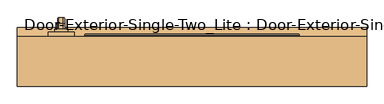
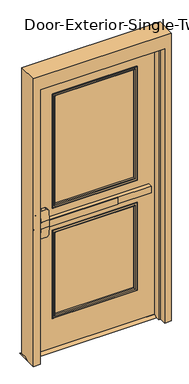
"""IFC4 building model written with IfcOpenShell, lengths in millimetres: door geometry, Door-Exterior-Single-Two_Lite : Door-Exterior-Single-Two_Lite."""

from ifc_helpers import new_model, si_unit, point, frame, frame_2d, origin, place, context, project, spatial, polyline, circle_curve, ellipse_curve, trimmed, segment, composite_curve, outline, extrude, faceted_brep, source, transform, mapped, element, save
from ifc_brep_helpers import plane_surface, cylinder_surface, revolved_surface, advanced_brep


def door_exterior_single_two_lite_door_exterior_single_two_lite_eb677f4d(model_context):
    return source(origin(), model_context, "Body", "SolidModel", [
        extrude(outline(polyline([(86.5, 12.7), (130.95, 12.7), (156.35, 0.0), (61.1, 0.0), (86.5, 12.7)])), frame((-508.0, 0.0, 0.0), z_axis=(1.0, 0.0, 0.0), x_axis=(0.0, 1.0, 0.0)), (0.0, 0.0, 1.0), 1016.0),
        extrude(outline(polyline([(150.2833333, 48.4), (-349.25, 48.4), (-349.25, 54.75), (150.2833333, 54.75), (150.2833333, 48.4)])), frame((0.0, 0.0, 990.6), z_axis=(0.0, 0.0, 1.0), x_axis=(1.0, 0.0, 0.0)), (0.0, 0.0, 1.0), 50.8),
        advanced_brep(
        [(-412.75, 54.75, 1041.4), (-412.75, 54.75, 990.6), (-349.25, 54.75, 990.6), (400.05, 54.75, 990.6), (400.05, 54.75, 1041.4), (-349.25, 54.75, 1041.4), (400.05, 86.5, 1041.4), (400.05, 86.5, 990.6), (-349.25, 86.5, 990.6), (-349.25, 86.5, 927.1), (-368.3, 86.5, 908.05), (-393.7, 86.5, 908.05), (-412.75, 86.5, 927.1), (-412.75, 86.5, 1104.9), (-393.7, 86.5, 1123.95), (-368.3, 86.5, 1123.95), (-349.25, 86.5, 1104.9), (-349.25, 86.5, 1041.4), (-349.25, 57.9252467, 1041.4), (-412.75, 57.9252467, 1041.4), (-412.75, 62.9354269, 1104.9), (-412.75, 62.9354269, 927.1), (-412.75, 57.9252467, 990.6), (-349.25, 57.9252467, 990.6), (-349.25, 62.9354269, 927.1), (-349.25, 62.9354269, 1104.9), (-393.7, 64.438481, 1123.95), (-368.3, 64.438481, 1123.95), (-368.3, 64.438481, 908.05), (-393.7, 64.438481, 908.05)],
        [
            (0, 1),
            (1, 2),
            (2, 3),
            (3, 4),
            (4, 5),
            (5, 0),
            (6, 7),
            (7, 8),
            (8, 9),
            (9, 10, circle_curve(frame((-368.3, 86.5, 927.1), z_axis=(0.0, 1.0, 0.0), x_axis=(1.0, 0.0, 0.0)), 19.05)),
            (10, 11),
            (11, 12, circle_curve(frame((-393.7, 86.5, 927.1), z_axis=(0.0, 1.0, 0.0), x_axis=(1.0, 0.0, 0.0)), 19.05)),
            (12, 13),
            (13, 14, circle_curve(frame((-393.7, 86.5, 1104.9), z_axis=(0.0, 1.0, 0.0), x_axis=(1.0, 0.0, 0.0)), 19.05)),
            (14, 15),
            (15, 16, circle_curve(frame((-368.3, 86.5, 1104.9), z_axis=(0.0, 1.0, 0.0), x_axis=(1.0, 0.0, 0.0)), 19.05)),
            (16, 17),
            (17, 6),
            (4, 6),
            (17, 18),
            (18, 19),
            (19, 0),
            (19, 20),
            (20, 13),
            (12, 21),
            (21, 22),
            (22, 1),
            (7, 3),
            (22, 23),
            (23, 8),
            (23, 24),
            (24, 9),
            (16, 25),
            (25, 18),
            (14, 26),
            (26, 27),
            (27, 15),
            (10, 28),
            (28, 29),
            (29, 11),
            (24, 28, ellipse_curve(frame((-368.3, 62.9354269, 927.1), z_axis=(0.0, 0.9969018152893365, 0.07865602756830282), x_axis=(0.0, -0.07865602756830208, 0.9969018152893365)), 19.1092038, 19.05)),
            (27, 25, ellipse_curve(frame((-368.3, 62.9354269, 1104.9), z_axis=(0.0, 0.9969018152893376, -0.07865602756828934), x_axis=(0.0, -0.078656027568288, -0.9969018152893377)), 19.1092038, 19.05)),
            (20, 26, ellipse_curve(frame((-393.7, 62.9354269, 1104.9), z_axis=(0.0, 0.9969018152893376, -0.07865602756828934), x_axis=(0.0, -0.078656027568288, -0.9969018152893377)), 19.1092038, 19.05)),
            (29, 21, ellipse_curve(frame((-393.7, 62.9354269, 927.1), z_axis=(0.0, 0.9969018152893365, 0.07865602756830282), x_axis=(0.0, -0.07865602756830208, 0.9969018152893365)), 19.1092038, 19.05)),
        ],
        [
            plane_surface(frame((-412.75, 54.75, 1041.4), z_axis=(0.0, -1.0, 0.0), x_axis=(-1.0, 0.0, 0.0))),
            plane_surface(frame((-412.75, 86.5, 1041.4), z_axis=(0.0, 1.0, 0.0), x_axis=(1.0, 0.0, 0.0))),
            plane_surface(frame((400.05, 54.75, 1041.4), z_axis=(0.0, 0.0, 1.0), x_axis=(0.0, 1.0, 0.0))),
            plane_surface(frame((-412.75, 54.75, 1041.4), z_axis=(-1.0, 0.0, 0.0), x_axis=(0.0, 1.0, 0.0))),
            plane_surface(frame((-412.75, 54.75, 990.6), z_axis=(0.0, 0.0, -1.0), x_axis=(0.0, 1.0, 0.0))),
            plane_surface(frame((400.05, 54.75, 990.6), z_axis=(1.0, 0.0, 0.0), x_axis=(0.0, 1.0, 0.0))),
            plane_surface(frame((-349.25, 57.9252467, 927.1), z_axis=(1.0, 0.0, 0.0), x_axis=(0.0, 1.0, 0.0))),
            plane_surface(frame((-368.3, 57.9252467, 1123.95), z_axis=(0.0, 0.0, 1.0), x_axis=(0.0, 1.0, 0.0))),
            plane_surface(frame((-393.7, 57.9252467, 908.05), z_axis=(0.0, 0.0, -1.0), x_axis=(0.0, 1.0, 0.0))),
            cylinder_surface(frame((-368.3, 86.5, 927.1), z_axis=(0.0, -1.0, 0.0), x_axis=(1.0, 0.0, 0.0)), 19.05),
            cylinder_surface(frame((-368.3, 86.5, 1104.9), z_axis=(0.0, -1.0, 0.0), x_axis=(1.0, 0.0, 0.0)), 19.05),
            cylinder_surface(frame((-393.7, 86.5, 1104.9), z_axis=(0.0, -1.0, 0.0), x_axis=(1.0, 0.0, 0.0)), 19.05),
            cylinder_surface(frame((-393.7, 86.5, 927.1), z_axis=(0.0, -1.0, 0.0), x_axis=(1.0, 0.0, 0.0)), 19.05),
            plane_surface(frame((-349.25, 57.9252467, 1041.4), z_axis=(0.0, -0.9969018152893376, 0.07865602756828934), x_axis=(-1.0, 0.0, 0.0))),
            plane_surface(frame((-349.25, 64.438481, 908.05), z_axis=(0.0, -0.9969018152893365, -0.07865602756830282), x_axis=(-1.0, 0.0, 0.0))),
        ],
        [
            (0, [[1, 2, 3, 4, 5, 6]]),
            (1, [[7, 8, 9, 10, 11, 12, 13, 14, 15, 16, 17, 18]]),
            (2, [[19, -18, 20, 21, 22, -6, -5]]),
            (3, [[-1, -22, 23, 24, -13, 25, 26, 27]]),
            (4, [[28, -3, -2, -27, 29, 30, -8]]),
            (5, [[-4, -28, -7, -19]]),
            (6, [[-9, -30, 31, 32]]),
            (6, [[-17, 33, 34, -20]]),
            (7, [[-15, 35, 36, 37]]),
            (8, [[-11, 38, 39, 40]]),
            (9, [[-10, -32, 41, -38]]),
            (10, [[-16, -37, 42, -33]]),
            (11, [[-14, -24, 43, -35]]),
            (12, [[-12, -40, 44, -25]]),
            (13, [[-21, -34, -42, -36, -43, -23]]),
            (14, [[-26, -44, -39, -41, -31, -29]]),
        ],
    ),
        advanced_brep(
        [(-391.0, 143.65, 1017.190625), (-391.0, 143.65, 1014.809375), (-387.428125, 143.65, 1011.2375), (-374.5715406, 143.65, 1011.2375), (-371.0, 143.65, 1014.8090406), (-371.0, 143.65, 1017.190625), (-374.571875, 143.65, 1020.7625), (-387.428125, 143.65, 1020.7625), (-391.0, 143.65, 887.809375), (-387.428125, 143.65, 884.2375), (-374.571875, 143.65, 884.2375), (-371.0, 143.65, 887.809375), (-371.0, 143.65, 890.1909594), (-374.5715406, 143.65, 893.7625), (-387.428125, 143.65, 893.7625), (-391.0, 143.65, 890.190625), (-391.0, 169.05, 1017.190625), (-391.0, 182.940625, 1003.3), (-391.0, 182.940625, 901.7), (-391.0, 169.05, 887.809375), (-391.0, 169.05, 890.190625), (-391.0, 180.559375, 901.7), (-391.0, 180.559375, 1003.3), (-391.0, 169.05, 1014.809375), (-387.428125, 169.05, 1011.2375), (-374.5715406, 169.05, 1011.2375), (-371.0, 169.05, 1014.8090406), (-371.0, 180.5590406, 1003.3), (-371.0, 180.5590406, 901.7), (-371.0, 169.05, 890.1909594), (-371.0, 169.05, 887.809375), (-371.0, 182.940625, 901.7), (-371.0, 182.940625, 1003.3), (-371.0, 169.05, 1017.190625), (-374.571875, 169.05, 1020.7625), (-387.428125, 169.05, 1020.7625), (-387.428125, 176.9875, 1003.3), (-374.5715406, 176.9875, 1003.3), (-374.571875, 186.5125, 1003.3), (-387.428125, 186.5125, 1003.3), (-387.428125, 176.9875, 901.7), (-374.5715406, 176.9875, 901.7), (-374.571875, 186.5125, 901.7), (-387.428125, 186.5125, 901.7), (-387.428125, 169.05, 893.7625), (-374.5715406, 169.05, 893.7625), (-374.571875, 169.05, 884.2375), (-387.428125, 169.05, 884.2375)],
        [
            (0, 1),
            (1, 2, circle_curve(frame((-387.428125, 143.65, 1014.809375), z_axis=(0.0, -1.0, 0.0), x_axis=(0.0, 0.0, 1.0)), 3.571875)),
            (2, 3),
            (3, 4, circle_curve(frame((-374.5715406, 143.65, 1014.8090406), z_axis=(0.0, -1.0, 0.0), x_axis=(0.0, 0.0, 1.0)), 3.5715406)),
            (4, 5),
            (5, 6, circle_curve(frame((-374.571875, 143.65, 1017.190625), z_axis=(0.0, -1.0, 0.0), x_axis=(0.0, 0.0, 1.0)), 3.571875)),
            (6, 7),
            (7, 0, circle_curve(frame((-387.428125, 143.65, 1017.190625), z_axis=(0.0, -1.0, 0.0), x_axis=(0.0, 0.0, 1.0)), 3.571875)),
            (8, 9, circle_curve(frame((-387.428125, 143.65, 887.809375), z_axis=(0.0, -1.0, 0.0), x_axis=(0.0, 0.0, -1.0)), 3.571875)),
            (9, 10),
            (10, 11, circle_curve(frame((-374.571875, 143.65, 887.809375), z_axis=(0.0, -1.0, 0.0), x_axis=(0.0, 0.0, -1.0)), 3.571875)),
            (11, 12),
            (12, 13, circle_curve(frame((-374.5715406, 143.65, 890.1909594), z_axis=(0.0, -1.0, 0.0), x_axis=(0.0, 0.0, -1.0)), 3.5715406)),
            (13, 14),
            (14, 15, circle_curve(frame((-387.428125, 143.65, 890.190625), z_axis=(0.0, -1.0, 0.0), x_axis=(0.0, 0.0, -1.0)), 3.571875)),
            (15, 8),
            (0, 16),
            (16, 17, circle_curve(frame((-391.0, 169.05, 1003.3), z_axis=(-1.0, 0.0, 0.0), x_axis=(0.0, 0.0, 1.0)), 13.890625)),
            (17, 18),
            (18, 19, circle_curve(frame((-391.0, 169.05, 901.7), z_axis=(-1.0, 0.0, 0.0), x_axis=(0.0, 1.0, 0.0)), 13.890625)),
            (19, 8),
            (15, 20),
            (20, 21, circle_curve(frame((-391.0, 169.05, 901.7), z_axis=(1.0, 0.0, 0.0), x_axis=(0.0, 1.0, 0.0)), 11.509375)),
            (21, 22),
            (22, 23, circle_curve(frame((-391.0, 169.05, 1003.3), z_axis=(1.0, 0.0, 0.0), x_axis=(0.0, 0.0, 1.0)), 11.509375)),
            (23, 1),
            (23, 24, circle_curve(frame((-387.428125, 169.05, 1014.809375), z_axis=(0.0, -1.0, 0.0), x_axis=(0.0, 0.0, 1.0)), 3.571875)),
            (24, 2),
            (24, 25),
            (25, 3),
            (25, 26, circle_curve(frame((-374.5715406, 169.05, 1014.8090406), z_axis=(0.0, -1.0, 0.0), x_axis=(0.0, 0.0, 1.0)), 3.5715406)),
            (26, 4),
            (26, 27, circle_curve(frame((-371.0, 169.05, 1003.3), z_axis=(-1.0, 0.0, 0.0), x_axis=(0.0, 0.0, 1.0)), 11.5090406)),
            (27, 28),
            (28, 29, circle_curve(frame((-371.0, 169.05, 901.7), z_axis=(-1.0, 0.0, 0.0), x_axis=(0.0, 1.0, 0.0)), 11.5090406)),
            (29, 12),
            (11, 30),
            (30, 31, circle_curve(frame((-371.0, 169.05, 901.7), z_axis=(1.0, 0.0, 0.0), x_axis=(0.0, 1.0, 0.0)), 13.890625)),
            (31, 32),
            (32, 33, circle_curve(frame((-371.0, 169.05, 1003.3), z_axis=(1.0, 0.0, 0.0), x_axis=(0.0, 0.0, 1.0)), 13.890625)),
            (33, 5),
            (33, 34, circle_curve(frame((-374.571875, 169.05, 1017.190625), z_axis=(0.0, -1.0, 0.0), x_axis=(0.0, 0.0, 1.0)), 3.571875)),
            (34, 6),
            (34, 35),
            (35, 7),
            (35, 16, circle_curve(frame((-387.428125, 169.05, 1017.190625), z_axis=(0.0, -1.0, 0.0), x_axis=(0.0, 0.0, 1.0)), 3.571875)),
            (36, 24, circle_curve(frame((-387.428125, 169.05, 1003.3), z_axis=(1.0, 0.0, 0.0), x_axis=(0.0, 0.0, 1.0)), 7.9375)),
            (22, 36, circle_curve(frame((-387.428125, 180.559375, 1003.3), z_axis=(0.0, 0.0, 1.0), x_axis=(0.0, 1.0, 0.0)), 3.571875)),
            (37, 25, circle_curve(frame((-374.5715406, 169.05, 1003.3), z_axis=(1.0, 0.0, 0.0), x_axis=(0.0, 0.0, 1.0)), 7.9375)),
            (36, 37),
            (37, 27, circle_curve(frame((-374.5715406, 180.5590406, 1003.3), z_axis=(0.0, 0.0, 1.0), x_axis=(0.0, 1.0, 0.0)), 3.5715406)),
            (38, 34, circle_curve(frame((-374.571875, 169.05, 1003.3), z_axis=(1.0, 0.0, 0.0), x_axis=(0.0, 0.0, 1.0)), 17.4625)),
            (32, 38, circle_curve(frame((-374.571875, 182.940625, 1003.3), z_axis=(0.0, 0.0, 1.0), x_axis=(0.0, 1.0, 0.0)), 3.571875)),
            (39, 35, circle_curve(frame((-387.428125, 169.05, 1003.3), z_axis=(1.0, 0.0, 0.0), x_axis=(0.0, 0.0, 1.0)), 17.4625)),
            (38, 39),
            (39, 17, circle_curve(frame((-387.428125, 182.940625, 1003.3), z_axis=(0.0, 0.0, 1.0), x_axis=(0.0, 1.0, 0.0)), 3.571875)),
            (21, 40, circle_curve(frame((-387.428125, 180.559375, 901.7), z_axis=(0.0, 0.0, 1.0), x_axis=(0.0, 1.0, 0.0)), 3.571875)),
            (40, 36),
            (40, 41),
            (41, 37),
            (41, 28, circle_curve(frame((-374.5715406, 180.5590406, 901.7), z_axis=(0.0, 0.0, 1.0), x_axis=(0.0, 1.0, 0.0)), 3.5715406)),
            (31, 42, circle_curve(frame((-374.571875, 182.940625, 901.7), z_axis=(0.0, 0.0, 1.0), x_axis=(0.0, 1.0, 0.0)), 3.571875)),
            (42, 38),
            (42, 43),
            (43, 39),
            (43, 18, circle_curve(frame((-387.428125, 182.940625, 901.7), z_axis=(0.0, 0.0, 1.0), x_axis=(0.0, 1.0, 0.0)), 3.571875)),
            (44, 40, circle_curve(frame((-387.428125, 169.05, 901.7), z_axis=(1.0, 0.0, 0.0), x_axis=(0.0, 1.0, 0.0)), 7.9375)),
            (20, 44, circle_curve(frame((-387.428125, 169.05, 890.190625), z_axis=(0.0, 1.0, 0.0), x_axis=(0.0, 0.0, -1.0)), 3.571875)),
            (45, 41, circle_curve(frame((-374.5715406, 169.05, 901.7), z_axis=(1.0, 0.0, 0.0), x_axis=(0.0, 1.0, 0.0)), 7.9375)),
            (44, 45),
            (45, 29, circle_curve(frame((-374.5715406, 169.05, 890.1909594), z_axis=(0.0, 1.0, 0.0), x_axis=(0.0, 0.0, -1.0)), 3.5715406)),
            (46, 42, circle_curve(frame((-374.571875, 169.05, 901.7), z_axis=(1.0, 0.0, 0.0), x_axis=(0.0, 1.0, 0.0)), 17.4625)),
            (30, 46, circle_curve(frame((-374.571875, 169.05, 887.809375), z_axis=(0.0, 1.0, 0.0), x_axis=(0.0, 0.0, -1.0)), 3.571875)),
            (47, 43, circle_curve(frame((-387.428125, 169.05, 901.7), z_axis=(1.0, 0.0, 0.0), x_axis=(0.0, 1.0, 0.0)), 17.4625)),
            (46, 47),
            (47, 19, circle_curve(frame((-387.428125, 169.05, 887.809375), z_axis=(0.0, 1.0, 0.0), x_axis=(0.0, 0.0, -1.0)), 3.571875)),
            (14, 44),
            (13, 45),
            (10, 46),
            (9, 47),
        ],
        [
            plane_surface(frame((-381.0, 143.65, 1016.0), z_axis=(0.0, -1.0, 0.0), x_axis=(1.0, 0.0, 0.0))),
            plane_surface(frame((-381.0, 143.65, 889.0), z_axis=(0.0, -1.0, 0.0), x_axis=(1.0, 0.0, 0.0))),
            plane_surface(frame((-391.0, 143.65, 1017.190625), z_axis=(-1.0, 0.0, 0.0), x_axis=(0.0, 1.0, 0.0))),
            cylinder_surface(frame((-387.428125, 143.65, 1014.809375), z_axis=(0.0, -1.0, 0.0), x_axis=(0.0, 0.0, 1.0)), 3.571875),
            plane_surface(frame((-387.428125, 143.65, 1011.2375), z_axis=(0.0, 0.0, -1.0), x_axis=(0.0, 1.0, 0.0))),
            cylinder_surface(frame((-374.5715406, 143.65, 1014.8090406), z_axis=(0.0, -1.0, 0.0), x_axis=(0.0, 0.0, 1.0)), 3.5715406),
            plane_surface(frame((-371.0, 143.65, 1014.8090406), z_axis=(1.0, 0.0, 0.0), x_axis=(0.0, 1.0, 0.0))),
            cylinder_surface(frame((-374.571875, 143.65, 1017.190625), z_axis=(0.0, -1.0, 0.0), x_axis=(0.0, 0.0, 1.0)), 3.571875),
            plane_surface(frame((-374.571875, 143.65, 1020.7625), z_axis=(0.0, 0.0, 1.0), x_axis=(0.0, 1.0, 0.0))),
            cylinder_surface(frame((-387.428125, 143.65, 1017.190625), z_axis=(0.0, -1.0, 0.0), x_axis=(0.0, 0.0, 1.0)), 3.571875),
            revolved_surface(trimmed(ellipse_curve(frame((-387.428125, 169.05, 1014.809375), z_axis=(0.0, -1.0, 0.0), x_axis=(0.0, 0.0, 1.0)), 3.571875, 3.571875), [point((-391.0, 169.05, 1014.809375))], [point((-387.428125, 169.05, 1011.2375))], True, "CARTESIAN"), (-381.0, 169.05, 1003.3), (-1.0, 0.0, 0.0)),
            revolved_surface(polyline([(-387.428125, 169.05, 1011.2375), (-374.5715406, 169.05, 1011.2375)]), (-381.0, 169.05, 1003.3), (-1.0, 0.0, 0.0)),
            revolved_surface(trimmed(ellipse_curve(frame((-374.5715406, 169.05, 1014.8090406), z_axis=(0.0, -1.0, 0.0), x_axis=(0.0, 0.0, 1.0)), 3.5715406, 3.5715406), [point((-374.5715406, 169.05, 1011.2375))], [point((-371.0, 169.05, 1014.8090406))], True, "CARTESIAN"), (-381.0, 169.05, 1003.3), (-1.0, 0.0, 0.0)),
            revolved_surface(trimmed(ellipse_curve(frame((-374.571875, 169.05, 1017.190625), z_axis=(0.0, -1.0, 0.0), x_axis=(0.0, 0.0, 1.0)), 3.571875, 3.571875), [point((-371.0, 169.05, 1017.190625))], [point((-374.571875, 169.05, 1020.7625))], True, "CARTESIAN"), (-381.0, 169.05, 1003.3), (-1.0, 0.0, 0.0)),
            cylinder_surface(frame((-381.0, 169.05, 1003.3), z_axis=(-1.0, 0.0, 0.0), x_axis=(0.0, 0.0, 1.0)), 17.4625),
            revolved_surface(trimmed(ellipse_curve(frame((-387.428125, 169.05, 1017.190625), z_axis=(0.0, -1.0, 0.0), x_axis=(0.0, 0.0, 1.0)), 3.571875, 3.571875), [point((-387.428125, 169.05, 1020.7625))], [point((-391.0, 169.05, 1017.190625))], True, "CARTESIAN"), (-381.0, 169.05, 1003.3), (-1.0, 0.0, 0.0)),
            cylinder_surface(frame((-387.428125, 180.559375, 1003.3), z_axis=(0.0, 0.0, 1.0), x_axis=(0.0, 1.0, 0.0)), 3.571875),
            plane_surface(frame((-387.428125, 176.9875, 1003.3), z_axis=(0.0, -1.0, 0.0), x_axis=(0.0, 0.0, -1.0))),
            cylinder_surface(frame((-374.5715406, 180.5590406, 1003.3), z_axis=(0.0, 0.0, 1.0), x_axis=(0.0, 1.0, 0.0)), 3.5715406),
            cylinder_surface(frame((-374.571875, 182.940625, 1003.3), z_axis=(0.0, 0.0, 1.0), x_axis=(0.0, 1.0, 0.0)), 3.571875),
            plane_surface(frame((-374.571875, 186.5125, 1003.3), z_axis=(0.0, 1.0, 0.0), x_axis=(0.0, 0.0, -1.0))),
            cylinder_surface(frame((-387.428125, 182.940625, 1003.3), z_axis=(0.0, 0.0, 1.0), x_axis=(0.0, 1.0, 0.0)), 3.571875),
            revolved_surface(trimmed(ellipse_curve(frame((-387.428125, 180.559375, 901.7), z_axis=(0.0, 0.0, 1.0), x_axis=(0.0, 1.0, 0.0)), 3.571875, 3.571875), [point((-391.0, 180.559375, 901.7))], [point((-387.428125, 176.9875, 901.7))], True, "CARTESIAN"), (-381.0, 169.05, 901.7), (-1.0, 0.0, 0.0)),
            revolved_surface(polyline([(-387.428125, 176.9875, 901.7), (-374.5715406, 176.9875, 901.7)]), (-381.0, 169.05, 901.7), (-1.0, 0.0, 0.0)),
            revolved_surface(trimmed(ellipse_curve(frame((-374.5715406, 180.5590406, 901.7), z_axis=(0.0, 0.0, 1.0), x_axis=(0.0, 1.0, 0.0)), 3.5715406, 3.5715406), [point((-374.5715406, 176.9875, 901.7))], [point((-371.0, 180.5590406, 901.7))], True, "CARTESIAN"), (-381.0, 169.05, 901.7), (-1.0, 0.0, 0.0)),
            revolved_surface(trimmed(ellipse_curve(frame((-374.571875, 182.940625, 901.7), z_axis=(0.0, 0.0, 1.0), x_axis=(0.0, 1.0, 0.0)), 3.571875, 3.571875), [point((-371.0, 182.940625, 901.7))], [point((-374.571875, 186.5125, 901.7))], True, "CARTESIAN"), (-381.0, 169.05, 901.7), (-1.0, 0.0, 0.0)),
            cylinder_surface(frame((-381.0, 169.05, 901.7), z_axis=(-1.0, 0.0, 0.0), x_axis=(0.0, 1.0, 0.0)), 17.4625),
            revolved_surface(trimmed(ellipse_curve(frame((-387.428125, 182.940625, 901.7), z_axis=(0.0, 0.0, 1.0), x_axis=(0.0, 1.0, 0.0)), 3.571875, 3.571875), [point((-387.428125, 186.5125, 901.7))], [point((-391.0, 182.940625, 901.7))], True, "CARTESIAN"), (-381.0, 169.05, 901.7), (-1.0, 0.0, 0.0)),
            cylinder_surface(frame((-387.428125, 169.05, 890.190625), z_axis=(0.0, 1.0, 0.0), x_axis=(0.0, 0.0, -1.0)), 3.571875),
            plane_surface(frame((-387.428125, 169.05, 893.7625), z_axis=(0.0, 0.0, 1.0), x_axis=(0.0, -1.0, 0.0))),
            cylinder_surface(frame((-374.5715406, 169.05, 890.1909594), z_axis=(0.0, 1.0, 0.0), x_axis=(0.0, 0.0, -1.0)), 3.5715406),
            cylinder_surface(frame((-374.571875, 169.05, 887.809375), z_axis=(0.0, 1.0, 0.0), x_axis=(0.0, 0.0, -1.0)), 3.571875),
            plane_surface(frame((-374.571875, 169.05, 884.2375), z_axis=(0.0, 0.0, -1.0), x_axis=(0.0, -1.0, 0.0))),
            cylinder_surface(frame((-387.428125, 169.05, 887.809375), z_axis=(0.0, 1.0, 0.0), x_axis=(0.0, 0.0, -1.0)), 3.571875),
        ],
        [
            (0, [[1, 2, 3, 4, 5, 6, 7, 8]]),
            (1, [[9, 10, 11, 12, 13, 14, 15, 16]]),
            (2, [[-1, 17, 18, 19, 20, 21, -16, 22, 23, 24, 25, 26]]),
            (3, [[-2, -26, 27, 28]]),
            (4, [[-3, -28, 29, 30]]),
            (5, [[-4, -30, 31, 32]]),
            (6, [[-5, -32, 33, 34, 35, 36, -12, 37, 38, 39, 40, 41]]),
            (7, [[-6, -41, 42, 43]]),
            (8, [[-7, -43, 44, 45]]),
            (9, [[-8, -45, 46, -17]]),
            (10, [[47, -27, -25, 48]]),
            (11, [[49, -29, -47, 50]]),
            (12, [[-33, -31, -49, 51]]),
            (13, [[52, -42, -40, 53]]),
            (14, [[54, -44, -52, 55]]),
            (15, [[-18, -46, -54, 56]]),
            (16, [[-48, -24, 57, 58]]),
            (17, [[-50, -58, 59, 60]]),
            (18, [[-51, -60, 61, -34]]),
            (19, [[-53, -39, 62, 63]]),
            (20, [[-55, -63, 64, 65]]),
            (21, [[-56, -65, 66, -19]]),
            (22, [[67, -57, -23, 68]]),
            (23, [[69, -59, -67, 70]]),
            (24, [[-35, -61, -69, 71]]),
            (25, [[72, -62, -38, 73]]),
            (26, [[74, -64, -72, 75]]),
            (27, [[-20, -66, -74, 76]]),
            (28, [[-68, -22, -15, 77]]),
            (29, [[-70, -77, -14, 78]]),
            (30, [[-71, -78, -13, -36]]),
            (31, [[-73, -37, -11, 79]]),
            (32, [[-75, -79, -10, 80]]),
            (33, [[-76, -80, -9, -21]]),
        ],
    ),
        extrude(outline(composite_curve([segment(trimmed(circle_curve(frame_2d((1117.6, -381.0)), 19.0), [point((1117.6, -400.0))], [point((1117.6, -362.0))], False, "CARTESIAN"), True, "CONTINUOUS"), segment(trimmed(circle_curve(frame_2d((1117.6, -381.0)), 19.0), [point((1117.6, -362.0))], [point((1117.6, -400.0))], False, "CARTESIAN"), True, "CONTINUOUS")], self_intersect=False)), frame((0.0, 143.65, 0.0), z_axis=(0.0, 1.0, 0.0), x_axis=(0.0, 0.0, 1.0)), (0.0, 0.0, 1.0), 8.73125),
        extrude(outline(composite_curve([segment(trimmed(circle_curve(frame_2d((1113.0338574, -381.0)), 89.3016225), [point((1193.8, -342.9))], [point((1193.8, -419.1))], False, "CARTESIAN"), True, "CONTINUOUS"), segment(polyline([(1193.8, -419.1), (838.2, -419.1)]), True, "CONTINUOUS"), segment(trimmed(circle_curve(frame_2d((918.9661426, -381.0)), 89.3016225), [point((838.2, -419.1))], [point((838.2, -342.9))], False, "CARTESIAN"), True, "CONTINUOUS"), segment(polyline([(838.2, -342.9), (1193.8, -342.9)]), True, "CONTINUOUS")], self_intersect=False)), frame((0.0, 130.95, 0.0), z_axis=(0.0, 1.0, 0.0), x_axis=(0.0, 0.0, 1.0)), (0.0, 0.0, 1.0), 12.7),
        extrude(outline(polyline([(2133.6, -457.2), (12.7, -457.2), (12.7, 457.2), (2133.6, 457.2), (2133.6, -457.2)]), holes=[polyline([(1981.2, -304.8), (1981.2, 304.8), (1111.25, 304.8), (1111.25, -304.8), (1981.2, -304.8)]), polyline([(920.75, -304.8), (920.75, 304.8), (254.0, 304.8), (254.0, -304.8), (920.75, -304.8)])]), frame((0.0, 86.5, 0.0), z_axis=(0.0, 1.0, 0.0), x_axis=(0.0, 0.0, 1.0)), (0.0, 0.0, 1.0), 44.45),
        faceted_brep([(457.2, 81.7375, 0.0), (457.2, 130.95, 0.0), (508.0, 130.95, 0.0), (508.0, -15.1, 0.0), (457.2, -15.1, 0.0), (457.2, 34.1125, 0.0), (441.325, 34.1125, 0.0), (441.325, 81.7375, 0.0), (457.2, 81.7375, 2133.6), (457.2, 130.95, 2133.6), (-457.2, 130.95, 2133.6), (-457.2, 130.95, 0.0), (-508.0, 130.95, 0.0), (-508.0, 130.95, 2235.2), (508.0, 130.95, 2235.2), (508.0, -15.1, 2235.2), (-508.0, -15.1, 2235.2), (-508.0, -15.1, 0.0), (-457.2, -15.1, 0.0), (-457.2, -15.1, 2133.6), (457.2, -15.1, 2133.6), (457.2, 34.1125, 2133.6), (-457.2, 34.1125, 2133.6), (-457.2, 34.1125, 0.0), (-441.325, 34.1125, 0.0), (-441.325, 34.1125, 2117.725), (441.325, 34.1125, 2117.725), (441.325, 81.7375, 2117.725), (-441.325, 81.7375, 2117.725), (-441.325, 81.7375, 0.0), (-457.2, 81.7375, 0.0), (-457.2, 81.7375, 2133.6)], [[[0, 1, 2, 3, 4, 5, 6, 7]], [[1, 0, 8, 9]], [[2, 1, 9, 10, 11, 12, 13, 14]], [[3, 2, 14, 15]], [[4, 3, 15, 16, 17, 18, 19, 20]], [[5, 4, 20, 21]], [[6, 5, 21, 22, 23, 24, 25, 26]], [[7, 6, 26, 27]], [[0, 7, 27, 28, 29, 30, 31, 8]], [[9, 8, 31, 10]], [[20, 19, 22, 21]], [[26, 25, 28, 27]], [[12, 11, 30, 29, 24, 23, 18, 17]], [[11, 10, 31, 30]], [[13, 12, 17, 16]], [[19, 18, 23, 22]], [[25, 24, 29, 28]], [[15, 14, 13, 16]]]),
        extrude(outline(polyline([(304.8, 99.2), (-304.8, 99.2), (-304.8, 118.25), (304.8, 118.25), (304.8, 99.2)])), frame((0.0, 0.0, 1111.25), z_axis=(0.0, 0.0, 1.0), x_axis=(1.0, 0.0, 0.0)), (0.0, 0.0, 1.0), 869.95),
        extrude(outline(polyline([(304.8, 99.2), (-304.8, 99.2), (-304.8, 118.25), (304.8, 118.25), (304.8, 99.2)])), frame((0.0, 0.0, 254.0), z_axis=(0.0, 0.0, 1.0), x_axis=(1.0, 0.0, 0.0)), (0.0, 0.0, 1.0), 666.75),
        advanced_brep(
        [(-304.8, 118.25, 1981.2), (-304.8, 130.95, 1981.2), (-304.8, 130.95, 1111.25), (-304.8, 118.25, 1111.25), (-292.8, 131.95, 1969.2), (-292.8, 118.25, 1969.2), (-292.8, 118.25, 1123.25), (-292.8, 131.95, 1123.25), (-297.8, 136.95, 1974.2), (-297.8, 136.95, 1118.25), (-312.8, 134.95, 1989.2), (-310.8, 136.95, 1987.2), (-310.8, 136.95, 1105.25), (-312.8, 134.95, 1103.25), (-312.8, 130.95, 1989.2), (-312.8, 130.95, 1103.25), (304.8, 130.95, 1111.25), (304.8, 118.25, 1111.25), (292.8, 118.25, 1123.25), (292.8, 131.95, 1123.25), (297.8, 136.95, 1118.25), (310.8, 136.95, 1105.25), (312.8, 134.95, 1103.25), (312.8, 130.95, 1103.25), (304.8, 130.95, 1981.2), (304.8, 118.25, 1981.2), (292.8, 118.25, 1969.2), (292.8, 131.95, 1969.2), (297.8, 136.95, 1974.2), (310.8, 136.95, 1987.2), (312.8, 134.95, 1989.2), (312.8, 130.95, 1989.2)],
        [
            (0, 1),
            (1, 2),
            (2, 3),
            (3, 0),
            (4, 5),
            (5, 6),
            (6, 7),
            (7, 4),
            (8, 4, ellipse_curve(frame((-297.8, 131.95, 1974.2), z_axis=(-0.7071067811865475, 0.0, -0.7071067811865475), x_axis=(-0.7071067811865474, 0.0, 0.7071067811865476)), 7.0710678, 5.0)),
            (7, 9, ellipse_curve(frame((-297.8, 131.95, 1118.25), z_axis=(-0.7071067811865475, 0.0, 0.7071067811865475), x_axis=(0.7071067811865474, 0.0, 0.7071067811865476)), 7.0710678, 5.0)),
            (9, 8),
            (10, 11, ellipse_curve(frame((-310.8, 134.95, 1987.2), z_axis=(-0.7071067811865475, 0.0, -0.7071067811865475), x_axis=(-0.7071067811865474, 0.0, 0.7071067811865476)), 2.8284271, 2.0)),
            (11, 12),
            (12, 13, ellipse_curve(frame((-310.8, 134.95, 1105.25), z_axis=(-0.7071067811865475, 0.0, 0.7071067811865475), x_axis=(0.7071067811865474, 0.0, 0.7071067811865476)), 2.8284271, 2.0)),
            (13, 10),
            (14, 10),
            (13, 15),
            (15, 14),
            (2, 16),
            (16, 17),
            (17, 3),
            (6, 18),
            (18, 19),
            (19, 7),
            (19, 20, ellipse_curve(frame((297.8, 131.95, 1118.25), z_axis=(-0.7071067811865475, 0.0, -0.7071067811865475), x_axis=(-0.7071067811865476, 0.0, 0.7071067811865474)), 7.0710678, 5.0)),
            (20, 9),
            (12, 21),
            (21, 22, ellipse_curve(frame((310.8, 134.95, 1105.25), z_axis=(-0.7071067811865475, 0.0, -0.7071067811865475), x_axis=(-0.7071067811865476, 0.0, 0.7071067811865474)), 2.8284271, 2.0)),
            (22, 13),
            (22, 23),
            (23, 15),
            (16, 24),
            (24, 25),
            (25, 17),
            (18, 26),
            (26, 27),
            (27, 19),
            (27, 28, ellipse_curve(frame((297.8, 131.95, 1974.2), z_axis=(0.7071067811865475, 0.0, -0.7071067811865475), x_axis=(-0.7071067811865474, 0.0, -0.7071067811865476)), 7.0710678, 5.0)),
            (28, 20),
            (21, 29),
            (29, 30, ellipse_curve(frame((310.8, 134.95, 1987.2), z_axis=(0.7071067811865475, 0.0, -0.7071067811865475), x_axis=(-0.7071067811865474, 0.0, -0.7071067811865476)), 2.8284271, 2.0)),
            (30, 22),
            (30, 31),
            (31, 23),
            (31, 14),
            (1, 24),
            (0, 25),
            (5, 26),
            (4, 27),
            (8, 28),
            (11, 29),
            (10, 30),
        ],
        [
            plane_surface(frame((-304.8, 130.95, 1981.2), z_axis=(-1.0, 0.0, 0.0), x_axis=(0.0, 0.0, -1.0))),
            plane_surface(frame((-292.8, 118.25, 1969.2), z_axis=(1.0, 0.0, 0.0), x_axis=(0.0, 0.0, -1.0))),
            cylinder_surface(frame((-297.8, 131.95, 1981.2), z_axis=(0.0, 0.0, 1.0), x_axis=(-1.0, 0.0, 0.0)), 5.0),
            cylinder_surface(frame((-310.8, 134.95, 1981.2), z_axis=(0.0, 0.0, 1.0), x_axis=(-1.0, 0.0, 0.0)), 2.0),
            plane_surface(frame((-312.8, 134.95, 1989.2), z_axis=(-1.0, 0.0, 0.0), x_axis=(0.0, 0.0, -1.0))),
            plane_surface(frame((-304.8, 130.95, 1111.25), z_axis=(0.0, 0.0, -1.0), x_axis=(1.0, 0.0, 0.0))),
            plane_surface(frame((-292.8, 118.25, 1123.25), z_axis=(0.0, 0.0, 1.0), x_axis=(1.0, 0.0, 0.0))),
            cylinder_surface(frame((-304.8, 131.95, 1118.25), z_axis=(-1.0, 0.0, 0.0), x_axis=(0.0, 0.0, -1.0)), 5.0),
            cylinder_surface(frame((-304.8, 134.95, 1105.25), z_axis=(-1.0, 0.0, 0.0), x_axis=(0.0, 0.0, -1.0)), 2.0),
            plane_surface(frame((-312.8, 134.95, 1103.25), z_axis=(0.0, 0.0, -1.0), x_axis=(1.0, 0.0, 0.0))),
            plane_surface(frame((304.8, 130.95, 1111.25), z_axis=(1.0, 0.0, 0.0), x_axis=(0.0, 0.0, 1.0))),
            plane_surface(frame((292.8, 118.25, 1123.25), z_axis=(-1.0, 0.0, 0.0), x_axis=(0.0, 0.0, 1.0))),
            cylinder_surface(frame((297.8, 131.95, 1111.25), z_axis=(0.0, 0.0, -1.0), x_axis=(1.0, 0.0, 0.0)), 5.0),
            cylinder_surface(frame((310.8, 134.95, 1111.25), z_axis=(0.0, 0.0, -1.0), x_axis=(1.0, 0.0, 0.0)), 2.0),
            plane_surface(frame((312.8, 134.95, 1103.25), z_axis=(1.0, 0.0, 0.0), x_axis=(0.0, 0.0, 1.0))),
            plane_surface(frame((312.8, 130.95, 1989.2), z_axis=(0.0, -1.0, 0.0), x_axis=(-1.0, 0.0, 0.0))),
            plane_surface(frame((304.8, 130.95, 1981.2), z_axis=(0.0, 0.0, 1.0), x_axis=(-1.0, 0.0, 0.0))),
            plane_surface(frame((304.8, 118.25, 1981.2), z_axis=(0.0, -1.0, 0.0), x_axis=(-1.0, 0.0, 0.0))),
            plane_surface(frame((292.8, 118.25, 1969.2), z_axis=(0.0, 0.0, -1.0), x_axis=(-1.0, 0.0, 0.0))),
            cylinder_surface(frame((304.8, 131.95, 1974.2), z_axis=(1.0, 0.0, 0.0), x_axis=(0.0, 0.0, 1.0)), 5.0),
            plane_surface(frame((297.8, 136.95, 1974.2), z_axis=(0.0, 1.0, 0.0), x_axis=(-1.0, 0.0, 0.0))),
            cylinder_surface(frame((304.8, 134.95, 1987.2), z_axis=(1.0, 0.0, 0.0), x_axis=(0.0, 0.0, 1.0)), 2.0),
            plane_surface(frame((312.8, 134.95, 1989.2), z_axis=(0.0, 0.0, 1.0), x_axis=(-1.0, 0.0, 0.0))),
        ],
        [
            (0, [[1, 2, 3, 4]]),
            (1, [[5, 6, 7, 8]]),
            (2, [[9, -8, 10, 11]]),
            (3, [[12, 13, 14, 15]]),
            (4, [[16, -15, 17, 18]]),
            (5, [[-3, 19, 20, 21]]),
            (6, [[-7, 22, 23, 24]]),
            (7, [[-10, -24, 25, 26]]),
            (8, [[-14, 27, 28, 29]]),
            (9, [[-17, -29, 30, 31]]),
            (10, [[-20, 32, 33, 34]]),
            (11, [[-23, 35, 36, 37]]),
            (12, [[-25, -37, 38, 39]]),
            (13, [[-28, 40, 41, 42]]),
            (14, [[-30, -42, 43, 44]]),
            (15, [[-31, -44, 45, -18], [46, -32, -19, -2]]),
            (16, [[-33, -46, -1, 47]]),
            (17, [[-21, -34, -47, -4], [48, -35, -22, -6]]),
            (18, [[-36, -48, -5, 49]]),
            (19, [[-38, -49, -9, 50]]),
            (20, [[51, -40, -27, -13], [-26, -39, -50, -11]]),
            (21, [[-41, -51, -12, 52]]),
            (22, [[-43, -52, -16, -45]]),
        ],
    ),
        advanced_brep(
        [(-304.8, 99.2, 1111.25), (-304.8, 86.5, 1111.25), (-304.8, 86.5, 1981.2), (-304.8, 99.2, 1981.2), (-292.8, 85.5, 1123.25), (-292.8, 99.2, 1123.25), (-292.8, 99.2, 1969.2), (-292.8, 85.5, 1969.2), (-297.8, 80.5, 1118.25), (-297.8, 80.5, 1974.2), (-312.8, 82.5, 1103.25), (-310.8, 80.5, 1105.25), (-310.8, 80.5, 1987.2), (-312.8, 82.5, 1989.2), (-312.8, 86.5, 1103.25), (-312.8, 86.5, 1989.2), (304.8, 86.5, 1981.2), (304.8, 99.2, 1981.2), (292.8, 99.2, 1969.2), (292.8, 85.5, 1969.2), (297.8, 80.5, 1974.2), (310.8, 80.5, 1987.2), (312.8, 82.5, 1989.2), (312.8, 86.5, 1989.2), (304.8, 86.5, 1111.25), (304.8, 99.2, 1111.25), (292.8, 99.2, 1123.25), (292.8, 85.5, 1123.25), (297.8, 80.5, 1118.25), (310.8, 80.5, 1105.25), (312.8, 82.5, 1103.25), (312.8, 86.5, 1103.25)],
        [
            (0, 1),
            (1, 2),
            (2, 3),
            (3, 0),
            (4, 5),
            (5, 6),
            (6, 7),
            (7, 4),
            (8, 4, ellipse_curve(frame((-297.8, 85.5, 1118.25), z_axis=(-0.7071067811865475, 0.0, 0.7071067811865475), x_axis=(-0.7071067811865474, 0.0, -0.7071067811865476)), 7.0710678, 5.0)),
            (7, 9, ellipse_curve(frame((-297.8, 85.5, 1974.2), z_axis=(-0.7071067811865475, 0.0, -0.7071067811865475), x_axis=(0.7071067811865474, 0.0, -0.7071067811865476)), 7.0710678, 5.0)),
            (9, 8),
            (10, 11, ellipse_curve(frame((-310.8, 82.5, 1105.25), z_axis=(-0.7071067811865475, 0.0, 0.7071067811865475), x_axis=(-0.7071067811865474, 0.0, -0.7071067811865476)), 2.8284271, 2.0)),
            (11, 12),
            (12, 13, ellipse_curve(frame((-310.8, 82.5, 1987.2), z_axis=(-0.7071067811865475, 0.0, -0.7071067811865475), x_axis=(0.7071067811865474, 0.0, -0.7071067811865476)), 2.8284271, 2.0)),
            (13, 10),
            (14, 10),
            (13, 15),
            (15, 14),
            (2, 16),
            (16, 17),
            (17, 3),
            (6, 18),
            (18, 19),
            (19, 7),
            (19, 20, ellipse_curve(frame((297.8, 85.5, 1974.2), z_axis=(-0.7071067811865475, 0.0, 0.7071067811865475), x_axis=(-0.7071067811865476, 0.0, -0.7071067811865474)), 7.0710678, 5.0)),
            (20, 9),
            (12, 21),
            (21, 22, ellipse_curve(frame((310.8, 82.5, 1987.2), z_axis=(-0.7071067811865475, 0.0, 0.7071067811865475), x_axis=(-0.7071067811865476, 0.0, -0.7071067811865474)), 2.8284271, 2.0)),
            (22, 13),
            (22, 23),
            (23, 15),
            (16, 24),
            (24, 25),
            (25, 17),
            (18, 26),
            (26, 27),
            (27, 19),
            (27, 28, ellipse_curve(frame((297.8, 85.5, 1118.25), z_axis=(0.7071067811865475, 0.0, 0.7071067811865475), x_axis=(-0.7071067811865474, 0.0, 0.7071067811865476)), 7.0710678, 5.0)),
            (28, 20),
            (21, 29),
            (29, 30, ellipse_curve(frame((310.8, 82.5, 1105.25), z_axis=(0.7071067811865475, 0.0, 0.7071067811865475), x_axis=(-0.7071067811865474, 0.0, 0.7071067811865476)), 2.8284271, 2.0)),
            (30, 22),
            (30, 31),
            (31, 23),
            (31, 14),
            (1, 24),
            (0, 25),
            (5, 26),
            (4, 27),
            (8, 28),
            (11, 29),
            (10, 30),
        ],
        [
            plane_surface(frame((-304.8, 86.5, 1111.25), z_axis=(-1.0, 0.0, 0.0), x_axis=(0.0, 0.0, 1.0))),
            plane_surface(frame((-292.8, 99.2, 1123.25), z_axis=(1.0, 0.0, 0.0), x_axis=(0.0, 0.0, 1.0))),
            cylinder_surface(frame((-297.8, 85.5, 1111.25), z_axis=(0.0, 0.0, -1.0), x_axis=(-1.0, 0.0, 0.0)), 5.0),
            cylinder_surface(frame((-310.8, 82.5, 1111.25), z_axis=(0.0, 0.0, -1.0), x_axis=(-1.0, 0.0, 0.0)), 2.0),
            plane_surface(frame((-312.8, 82.5, 1103.25), z_axis=(-1.0, 0.0, 0.0), x_axis=(0.0, 0.0, 1.0))),
            plane_surface(frame((-304.8, 86.5, 1981.2), z_axis=(0.0, 0.0, 1.0), x_axis=(1.0, 0.0, 0.0))),
            plane_surface(frame((-292.8, 99.2, 1969.2), z_axis=(0.0, 0.0, -1.0), x_axis=(1.0, 0.0, 0.0))),
            cylinder_surface(frame((-304.8, 85.5, 1974.2), z_axis=(-1.0, 0.0, 0.0), x_axis=(0.0, 0.0, 1.0)), 5.0),
            cylinder_surface(frame((-304.8, 82.5, 1987.2), z_axis=(-1.0, 0.0, 0.0), x_axis=(0.0, 0.0, 1.0)), 2.0),
            plane_surface(frame((-312.8, 82.5, 1989.2), z_axis=(0.0, 0.0, 1.0), x_axis=(1.0, 0.0, 0.0))),
            plane_surface(frame((304.8, 86.5, 1981.2), z_axis=(1.0, 0.0, 0.0), x_axis=(0.0, 0.0, -1.0))),
            plane_surface(frame((292.8, 99.2, 1969.2), z_axis=(-1.0, 0.0, 0.0), x_axis=(0.0, 0.0, -1.0))),
            cylinder_surface(frame((297.8, 85.5, 1981.2), z_axis=(0.0, 0.0, 1.0), x_axis=(1.0, 0.0, 0.0)), 5.0),
            cylinder_surface(frame((310.8, 82.5, 1981.2), z_axis=(0.0, 0.0, 1.0), x_axis=(1.0, 0.0, 0.0)), 2.0),
            plane_surface(frame((312.8, 82.5, 1989.2), z_axis=(1.0, 0.0, 0.0), x_axis=(0.0, 0.0, -1.0))),
            plane_surface(frame((312.8, 86.5, 1103.25), z_axis=(0.0, 1.0, 0.0), x_axis=(-1.0, 0.0, 0.0))),
            plane_surface(frame((304.8, 86.5, 1111.25), z_axis=(0.0, 0.0, -1.0), x_axis=(-1.0, 0.0, 0.0))),
            plane_surface(frame((304.8, 99.2, 1111.25), z_axis=(0.0, 1.0, 0.0), x_axis=(-1.0, 0.0, 0.0))),
            plane_surface(frame((292.8, 99.2, 1123.25), z_axis=(0.0, 0.0, 1.0), x_axis=(-1.0, 0.0, 0.0))),
            cylinder_surface(frame((304.8, 85.5, 1118.25), z_axis=(1.0, 0.0, 0.0), x_axis=(0.0, 0.0, -1.0)), 5.0),
            plane_surface(frame((297.8, 80.5, 1118.25), z_axis=(0.0, -1.0, 0.0), x_axis=(-1.0, 0.0, 0.0))),
            cylinder_surface(frame((304.8, 82.5, 1105.25), z_axis=(1.0, 0.0, 0.0), x_axis=(0.0, 0.0, -1.0)), 2.0),
            plane_surface(frame((312.8, 82.5, 1103.25), z_axis=(0.0, 0.0, -1.0), x_axis=(-1.0, 0.0, 0.0))),
        ],
        [
            (0, [[1, 2, 3, 4]]),
            (1, [[5, 6, 7, 8]]),
            (2, [[9, -8, 10, 11]]),
            (3, [[12, 13, 14, 15]]),
            (4, [[16, -15, 17, 18]]),
            (5, [[-3, 19, 20, 21]]),
            (6, [[-7, 22, 23, 24]]),
            (7, [[-10, -24, 25, 26]]),
            (8, [[-14, 27, 28, 29]]),
            (9, [[-17, -29, 30, 31]]),
            (10, [[-20, 32, 33, 34]]),
            (11, [[-23, 35, 36, 37]]),
            (12, [[-25, -37, 38, 39]]),
            (13, [[-28, 40, 41, 42]]),
            (14, [[-30, -42, 43, 44]]),
            (15, [[-31, -44, 45, -18], [46, -32, -19, -2]]),
            (16, [[-33, -46, -1, 47]]),
            (17, [[-21, -34, -47, -4], [48, -35, -22, -6]]),
            (18, [[-36, -48, -5, 49]]),
            (19, [[-38, -49, -9, 50]]),
            (20, [[51, -40, -27, -13], [-26, -39, -50, -11]]),
            (21, [[-41, -51, -12, 52]]),
            (22, [[-43, -52, -16, -45]]),
        ],
    ),
        advanced_brep(
        [(-304.8, 118.25, 920.75), (-304.8, 130.95, 920.75), (-304.8, 130.95, 254.0), (-304.8, 118.25, 254.0), (-292.8, 131.95, 908.75), (-292.8, 118.25, 908.75), (-292.8, 118.25, 266.0), (-292.8, 131.95, 266.0), (-297.8, 136.95, 913.75), (-297.8, 136.95, 261.0), (-312.8, 134.95, 928.75), (-310.8, 136.95, 926.75), (-310.8, 136.95, 248.0), (-312.8, 134.95, 246.0), (-312.8, 130.95, 928.75), (-312.8, 130.95, 246.0), (304.8, 130.95, 254.0), (304.8, 118.25, 254.0), (292.8, 118.25, 266.0), (292.8, 131.95, 266.0), (297.8, 136.95, 261.0), (310.8, 136.95, 248.0), (312.8, 134.95, 246.0), (312.8, 130.95, 246.0), (304.8, 130.95, 920.75), (304.8, 118.25, 920.75), (292.8, 118.25, 908.75), (292.8, 131.95, 908.75), (297.8, 136.95, 913.75), (310.8, 136.95, 926.75), (312.8, 134.95, 928.75), (312.8, 130.95, 928.75)],
        [
            (0, 1),
            (1, 2),
            (2, 3),
            (3, 0),
            (4, 5),
            (5, 6),
            (6, 7),
            (7, 4),
            (8, 4, ellipse_curve(frame((-297.8, 131.95, 913.75), z_axis=(-0.7071067811865475, 0.0, -0.7071067811865475), x_axis=(-0.7071067811865474, 0.0, 0.7071067811865476)), 7.0710678, 5.0)),
            (7, 9, ellipse_curve(frame((-297.8, 131.95, 261.0), z_axis=(-0.7071067811865475, 0.0, 0.7071067811865475), x_axis=(0.7071067811865474, 0.0, 0.7071067811865476)), 7.0710678, 5.0)),
            (9, 8),
            (10, 11, ellipse_curve(frame((-310.8, 134.95, 926.75), z_axis=(-0.7071067811865475, 0.0, -0.7071067811865475), x_axis=(-0.7071067811865474, 0.0, 0.7071067811865476)), 2.8284271, 2.0)),
            (11, 12),
            (12, 13, ellipse_curve(frame((-310.8, 134.95, 248.0), z_axis=(-0.7071067811865475, 0.0, 0.7071067811865475), x_axis=(0.7071067811865474, 0.0, 0.7071067811865476)), 2.8284271, 2.0)),
            (13, 10),
            (14, 10),
            (13, 15),
            (15, 14),
            (2, 16),
            (16, 17),
            (17, 3),
            (6, 18),
            (18, 19),
            (19, 7),
            (19, 20, ellipse_curve(frame((297.8, 131.95, 261.0), z_axis=(-0.7071067811865475, 0.0, -0.7071067811865475), x_axis=(-0.7071067811865476, 0.0, 0.7071067811865474)), 7.0710678, 5.0)),
            (20, 9),
            (12, 21),
            (21, 22, ellipse_curve(frame((310.8, 134.95, 248.0), z_axis=(-0.7071067811865475, 0.0, -0.7071067811865475), x_axis=(-0.7071067811865476, 0.0, 0.7071067811865474)), 2.8284271, 2.0)),
            (22, 13),
            (22, 23),
            (23, 15),
            (16, 24),
            (24, 25),
            (25, 17),
            (18, 26),
            (26, 27),
            (27, 19),
            (27, 28, ellipse_curve(frame((297.8, 131.95, 913.75), z_axis=(0.7071067811865475, 0.0, -0.7071067811865475), x_axis=(-0.7071067811865474, 0.0, -0.7071067811865476)), 7.0710678, 5.0)),
            (28, 20),
            (21, 29),
            (29, 30, ellipse_curve(frame((310.8, 134.95, 926.75), z_axis=(0.7071067811865475, 0.0, -0.7071067811865475), x_axis=(-0.7071067811865474, 0.0, -0.7071067811865476)), 2.8284271, 2.0)),
            (30, 22),
            (30, 31),
            (31, 23),
            (31, 14),
            (1, 24),
            (0, 25),
            (5, 26),
            (4, 27),
            (8, 28),
            (11, 29),
            (10, 30),
        ],
        [
            plane_surface(frame((-304.8, 130.95, 920.75), z_axis=(-1.0, 0.0, 0.0), x_axis=(0.0, 0.0, -1.0))),
            plane_surface(frame((-292.8, 118.25, 908.75), z_axis=(1.0, 0.0, 0.0), x_axis=(0.0, 0.0, -1.0))),
            cylinder_surface(frame((-297.8, 131.95, 920.75), z_axis=(0.0, 0.0, 1.0), x_axis=(-1.0, 0.0, 0.0)), 5.0),
            cylinder_surface(frame((-310.8, 134.95, 920.75), z_axis=(0.0, 0.0, 1.0), x_axis=(-1.0, 0.0, 0.0)), 2.0),
            plane_surface(frame((-312.8, 134.95, 928.75), z_axis=(-1.0, 0.0, 0.0), x_axis=(0.0, 0.0, -1.0))),
            plane_surface(frame((-304.8, 130.95, 254.0), z_axis=(0.0, 0.0, -1.0), x_axis=(1.0, 0.0, 0.0))),
            plane_surface(frame((-292.8, 118.25, 266.0), z_axis=(0.0, 0.0, 1.0), x_axis=(1.0, 0.0, 0.0))),
            cylinder_surface(frame((-304.8, 131.95, 261.0), z_axis=(-1.0, 0.0, 0.0), x_axis=(0.0, 0.0, -1.0)), 5.0),
            cylinder_surface(frame((-304.8, 134.95, 248.0), z_axis=(-1.0, 0.0, 0.0), x_axis=(0.0, 0.0, -1.0)), 2.0),
            plane_surface(frame((-312.8, 134.95, 246.0), z_axis=(0.0, 0.0, -1.0), x_axis=(1.0, 0.0, 0.0))),
            plane_surface(frame((304.8, 130.95, 254.0), z_axis=(1.0, 0.0, 0.0), x_axis=(0.0, 0.0, 1.0))),
            plane_surface(frame((292.8, 118.25, 266.0), z_axis=(-1.0, 0.0, 0.0), x_axis=(0.0, 0.0, 1.0))),
            cylinder_surface(frame((297.8, 131.95, 254.0), z_axis=(0.0, 0.0, -1.0), x_axis=(1.0, 0.0, 0.0)), 5.0),
            cylinder_surface(frame((310.8, 134.95, 254.0), z_axis=(0.0, 0.0, -1.0), x_axis=(1.0, 0.0, 0.0)), 2.0),
            plane_surface(frame((312.8, 134.95, 246.0), z_axis=(1.0, 0.0, 0.0), x_axis=(0.0, 0.0, 1.0))),
            plane_surface(frame((312.8, 130.95, 928.75), z_axis=(0.0, -1.0, 0.0), x_axis=(-1.0, 0.0, 0.0))),
            plane_surface(frame((304.8, 130.95, 920.75), z_axis=(0.0, 0.0, 1.0), x_axis=(-1.0, 0.0, 0.0))),
            plane_surface(frame((304.8, 118.25, 920.75), z_axis=(0.0, -1.0, 0.0), x_axis=(-1.0, 0.0, 0.0))),
            plane_surface(frame((292.8, 118.25, 908.75), z_axis=(0.0, 0.0, -1.0), x_axis=(-1.0, 0.0, 0.0))),
            cylinder_surface(frame((304.8, 131.95, 913.75), z_axis=(1.0, 0.0, 0.0), x_axis=(0.0, 0.0, 1.0)), 5.0),
            plane_surface(frame((297.8, 136.95, 913.75), z_axis=(0.0, 1.0, 0.0), x_axis=(-1.0, 0.0, 0.0))),
            cylinder_surface(frame((304.8, 134.95, 926.75), z_axis=(1.0, 0.0, 0.0), x_axis=(0.0, 0.0, 1.0)), 2.0),
            plane_surface(frame((312.8, 134.95, 928.75), z_axis=(0.0, 0.0, 1.0), x_axis=(-1.0, 0.0, 0.0))),
        ],
        [
            (0, [[1, 2, 3, 4]]),
            (1, [[5, 6, 7, 8]]),
            (2, [[9, -8, 10, 11]]),
            (3, [[12, 13, 14, 15]]),
            (4, [[16, -15, 17, 18]]),
            (5, [[-3, 19, 20, 21]]),
            (6, [[-7, 22, 23, 24]]),
            (7, [[-10, -24, 25, 26]]),
            (8, [[-14, 27, 28, 29]]),
            (9, [[-17, -29, 30, 31]]),
            (10, [[-20, 32, 33, 34]]),
            (11, [[-23, 35, 36, 37]]),
            (12, [[-25, -37, 38, 39]]),
            (13, [[-28, 40, 41, 42]]),
            (14, [[-30, -42, 43, 44]]),
            (15, [[-31, -44, 45, -18], [46, -32, -19, -2]]),
            (16, [[-33, -46, -1, 47]]),
            (17, [[-21, -34, -47, -4], [48, -35, -22, -6]]),
            (18, [[-36, -48, -5, 49]]),
            (19, [[-38, -49, -9, 50]]),
            (20, [[51, -40, -27, -13], [-26, -39, -50, -11]]),
            (21, [[-41, -51, -12, 52]]),
            (22, [[-43, -52, -16, -45]]),
        ],
    ),
        advanced_brep(
        [(304.8, 99.2, 920.75), (304.8, 86.5, 920.75), (304.8, 86.5, 254.0), (304.8, 99.2, 254.0), (292.8, 85.5, 908.75), (292.8, 99.2, 908.75), (292.8, 99.2, 266.0), (292.8, 85.5, 266.0), (297.8, 80.5, 913.75), (297.8, 80.5, 261.0), (312.8, 82.5, 928.75), (310.8, 80.5, 926.75), (310.8, 80.5, 248.0), (312.8, 82.5, 246.0), (312.8, 86.5, 928.75), (312.8, 86.5, 246.0), (-304.8, 86.5, 254.0), (-304.8, 99.2, 254.0), (-292.8, 99.2, 266.0), (-292.8, 85.5, 266.0), (-297.8, 80.5, 261.0), (-310.8, 80.5, 248.0), (-312.8, 82.5, 246.0), (-312.8, 86.5, 246.0), (-304.8, 86.5, 920.75), (-304.8, 99.2, 920.75), (-292.8, 99.2, 908.75), (-292.8, 85.5, 908.75), (-297.8, 80.5, 913.75), (-310.8, 80.5, 926.75), (-312.8, 82.5, 928.75), (-312.8, 86.5, 928.75)],
        [
            (0, 1),
            (1, 2),
            (2, 3),
            (3, 0),
            (4, 5),
            (5, 6),
            (6, 7),
            (7, 4),
            (8, 4, ellipse_curve(frame((297.8, 85.5, 913.75), z_axis=(0.7071067811865475, 0.0, -0.7071067811865475), x_axis=(0.7071067811865474, 0.0, 0.7071067811865476)), 7.0710678, 5.0)),
            (7, 9, ellipse_curve(frame((297.8, 85.5, 261.0), z_axis=(0.7071067811865475, 0.0, 0.7071067811865475), x_axis=(-0.7071067811865474, 0.0, 0.7071067811865476)), 7.0710678, 5.0)),
            (9, 8),
            (10, 11, ellipse_curve(frame((310.8, 82.5, 926.75), z_axis=(0.7071067811865475, 0.0, -0.7071067811865475), x_axis=(0.7071067811865474, 0.0, 0.7071067811865476)), 2.8284271, 2.0)),
            (11, 12),
            (12, 13, ellipse_curve(frame((310.8, 82.5, 248.0), z_axis=(0.7071067811865475, 0.0, 0.7071067811865475), x_axis=(-0.7071067811865474, 0.0, 0.7071067811865476)), 2.8284271, 2.0)),
            (13, 10),
            (14, 10),
            (13, 15),
            (15, 14),
            (2, 16),
            (16, 17),
            (17, 3),
            (6, 18),
            (18, 19),
            (19, 7),
            (19, 20, ellipse_curve(frame((-297.8, 85.5, 261.0), z_axis=(0.7071067811865475, 0.0, -0.7071067811865475), x_axis=(0.7071067811865476, 0.0, 0.7071067811865474)), 7.0710678, 5.0)),
            (20, 9),
            (12, 21),
            (21, 22, ellipse_curve(frame((-310.8, 82.5, 248.0), z_axis=(0.7071067811865475, 0.0, -0.7071067811865475), x_axis=(0.7071067811865476, 0.0, 0.7071067811865474)), 2.8284271, 2.0)),
            (22, 13),
            (22, 23),
            (23, 15),
            (16, 24),
            (24, 25),
            (25, 17),
            (18, 26),
            (26, 27),
            (27, 19),
            (27, 28, ellipse_curve(frame((-297.8, 85.5, 913.75), z_axis=(-0.7071067811865475, 0.0, -0.7071067811865475), x_axis=(0.7071067811865474, 0.0, -0.7071067811865476)), 7.0710678, 5.0)),
            (28, 20),
            (21, 29),
            (29, 30, ellipse_curve(frame((-310.8, 82.5, 926.75), z_axis=(-0.7071067811865475, 0.0, -0.7071067811865475), x_axis=(0.7071067811865474, 0.0, -0.7071067811865476)), 2.8284271, 2.0)),
            (30, 22),
            (30, 31),
            (31, 23),
            (31, 14),
            (1, 24),
            (0, 25),
            (5, 26),
            (4, 27),
            (8, 28),
            (11, 29),
            (10, 30),
        ],
        [
            plane_surface(frame((304.8, 86.5, 920.75), z_axis=(1.0, 0.0, 0.0), x_axis=(0.0, 0.0, -1.0))),
            plane_surface(frame((292.8, 99.2, 908.75), z_axis=(-1.0, 0.0, 0.0), x_axis=(0.0, 0.0, -1.0))),
            cylinder_surface(frame((297.8, 85.5, 920.75), z_axis=(0.0, 0.0, 1.0), x_axis=(1.0, 0.0, 0.0)), 5.0),
            cylinder_surface(frame((310.8, 82.5, 920.75), z_axis=(0.0, 0.0, 1.0), x_axis=(1.0, 0.0, 0.0)), 2.0),
            plane_surface(frame((312.8, 82.5, 928.75), z_axis=(1.0, 0.0, 0.0), x_axis=(0.0, 0.0, -1.0))),
            plane_surface(frame((304.8, 86.5, 254.0), z_axis=(0.0, 0.0, -1.0), x_axis=(-1.0, 0.0, 0.0))),
            plane_surface(frame((292.8, 99.2, 266.0), z_axis=(0.0, 0.0, 1.0), x_axis=(-1.0, 0.0, 0.0))),
            cylinder_surface(frame((304.8, 85.5, 261.0), z_axis=(1.0, 0.0, 0.0), x_axis=(0.0, 0.0, -1.0)), 5.0),
            cylinder_surface(frame((304.8, 82.5, 248.0), z_axis=(1.0, 0.0, 0.0), x_axis=(0.0, 0.0, -1.0)), 2.0),
            plane_surface(frame((312.8, 82.5, 246.0), z_axis=(0.0, 0.0, -1.0), x_axis=(-1.0, 0.0, 0.0))),
            plane_surface(frame((-304.8, 86.5, 254.0), z_axis=(-1.0, 0.0, 0.0), x_axis=(0.0, 0.0, 1.0))),
            plane_surface(frame((-292.8, 99.2, 266.0), z_axis=(1.0, 0.0, 0.0), x_axis=(0.0, 0.0, 1.0))),
            cylinder_surface(frame((-297.8, 85.5, 254.0), z_axis=(0.0, 0.0, -1.0), x_axis=(-1.0, 0.0, 0.0)), 5.0),
            cylinder_surface(frame((-310.8, 82.5, 254.0), z_axis=(0.0, 0.0, -1.0), x_axis=(-1.0, 0.0, 0.0)), 2.0),
            plane_surface(frame((-312.8, 82.5, 246.0), z_axis=(-1.0, 0.0, 0.0), x_axis=(0.0, 0.0, 1.0))),
            plane_surface(frame((-312.8, 86.5, 928.75), z_axis=(0.0, 1.0, 0.0), x_axis=(1.0, 0.0, 0.0))),
            plane_surface(frame((-304.8, 86.5, 920.75), z_axis=(0.0, 0.0, 1.0), x_axis=(1.0, 0.0, 0.0))),
            plane_surface(frame((-304.8, 99.2, 920.75), z_axis=(0.0, 1.0, 0.0), x_axis=(1.0, 0.0, 0.0))),
            plane_surface(frame((-292.8, 99.2, 908.75), z_axis=(0.0, 0.0, -1.0), x_axis=(1.0, 0.0, 0.0))),
            cylinder_surface(frame((-304.8, 85.5, 913.75), z_axis=(-1.0, 0.0, 0.0), x_axis=(0.0, 0.0, 1.0)), 5.0),
            plane_surface(frame((-297.8, 80.5, 913.75), z_axis=(0.0, -1.0, 0.0), x_axis=(1.0, 0.0, 0.0))),
            cylinder_surface(frame((-304.8, 82.5, 926.75), z_axis=(-1.0, 0.0, 0.0), x_axis=(0.0, 0.0, 1.0)), 2.0),
            plane_surface(frame((-312.8, 82.5, 928.75), z_axis=(0.0, 0.0, 1.0), x_axis=(1.0, 0.0, 0.0))),
        ],
        [
            (0, [[1, 2, 3, 4]]),
            (1, [[5, 6, 7, 8]]),
            (2, [[9, -8, 10, 11]]),
            (3, [[12, 13, 14, 15]]),
            (4, [[16, -15, 17, 18]]),
            (5, [[-3, 19, 20, 21]]),
            (6, [[-7, 22, 23, 24]]),
            (7, [[-10, -24, 25, 26]]),
            (8, [[-14, 27, 28, 29]]),
            (9, [[-17, -29, 30, 31]]),
            (10, [[-20, 32, 33, 34]]),
            (11, [[-23, 35, 36, 37]]),
            (12, [[-25, -37, 38, 39]]),
            (13, [[-28, 40, 41, 42]]),
            (14, [[-30, -42, 43, 44]]),
            (15, [[-31, -44, 45, -18], [46, -32, -19, -2]]),
            (16, [[-33, -46, -1, 47]]),
            (17, [[-21, -34, -47, -4], [48, -35, -22, -6]]),
            (18, [[-36, -48, -5, 49]]),
            (19, [[-38, -49, -9, 50]]),
            (20, [[51, -40, -27, -13], [-26, -39, -50, -11]]),
            (21, [[-41, -51, -12, 52]]),
            (22, [[-43, -52, -16, -45]]),
        ],
    ),
    ])


if __name__ == "__main__":
    model = new_model("IFC4")
    model_context = context("Model", 3, world=origin())
    ifc_project = project(units=[si_unit("LENGTHUNIT", "METRE", prefix="MILLI")], contexts=[model_context])
    site = spatial("IfcSite", under=ifc_project)
    building = spatial("IfcBuilding", under=site)
    placement = place(None, origin())
    door_exterior_single_two_lite_door_exterior_single_two_lite_shape = door_exterior_single_two_lite_door_exterior_single_two_lite_eb677f4d(model_context)
    element("IfcDoor", 1, ObjectType="Door-Exterior-Single-Two_Lite : Door-Exterior-Single-Two_Lite", at=placement, inside=building, context=model_context, shape_type="MappedRepresentation", body=[
        mapped(door_exterior_single_two_lite_door_exterior_single_two_lite_shape, transform((0.0, 0.0, 0.0), x_axis=(1.0, 0.0, 0.0), y_axis=(0.0, 1.0, 0.0), z_axis=(0.0, 0.0, 1.0))),
    ])
    save(model, "model.ifc")

# Revit data of these elements
# Type "Door-Exterior-Single-Two_Lite : Door-Exterior-Single-Two_Lite"
#   Type Mark = "46"
#   Assembly Code = "B2030100"
#   Analytic Construction = "Metal frame, double glass door"
#   Top Rail = 152.4 mm
#   Threshold Offset [instance default] = 12.7 mm
#   Threshold Length [instance default] = 1016 mm
#   Thickness = 44.45 mm
#   Thermal Resistance (R) = 0.242926 (m²·K)/W
#   Swing Angle [instance default] = 90.00°
#   Strike Height = 1016 mm
#   Stiles = 152.4 mm
#   Rough Width [instance default] = 1016 mm
#   Rough Height [instance default] = 2235.2 mm
#   MFOpeningHeight [instance default] = 101.6 mm
#   MFOpeningWidth [instance default] = 101.6 mm
#   Lock Rail = 190.5 mm
#   Heat Transfer Coefficient (U) = 4.11674 W/(m²·K)
#   Glass Thickness = 19.05 mm
#   Inset Calculate [instance default] = 101.6 mm
#   Masonry Inset [instance default] = 25.4 mm
#   Height = 2133.6 mm
#   Width = 914.4 mm
#   Masonry Frame Depth = 146.05 mm
#   Bottom Rail = 254 mm
#   Masonry Frame [instance default] = yes
#   Function = 1
#   Threshold [instance default] = yes
#   Dry Wall Frame [instance default] = no
#   Threshold Material = none
#   Panic Bar Material = Metal - Stainless Steel
#   Panel Material = Metal - Painted - Grey
#   Glass Stop Material = Metal - Painted - Grey
#   Exterior Pull Material = Metal - Stainless Steel
#   Frame Material = Metal - Painted - Grey
#   Visual Light Transmittance = 0
#   Solar Heat Gain Coefficient = 0
#   Wall Closure = (empty or 0)
# Element 1 (IfcDoor, "Door-Exterior-Single-Two_Lite : Door-Exterior-Single-Two_Lite")
#   Materials on its faces: "Metal - Painted - Grey", "Metal - Stainless Steel", "Glass", "Door - Frame/Mullion"
# Materials
#   "Metal - Stainless Steel": class "Metal", colour RGB 247 247 247, transparency 0
#   "Metal - Painted - Grey": class "Paint", colour RGB 104 104 104, transparency 0
#   "Glass": class "Glass", colour RGB 0 128 192, transparency 0.9, Description = "Soda Lime Glass", Cost = 0
#   "Door - Frame/Mullion": class "Wood", colour RGB 212 179 113, transparency 0, Keynote = "L20", Cost = 0
